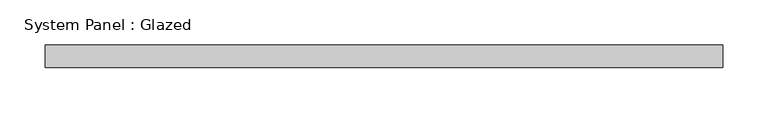
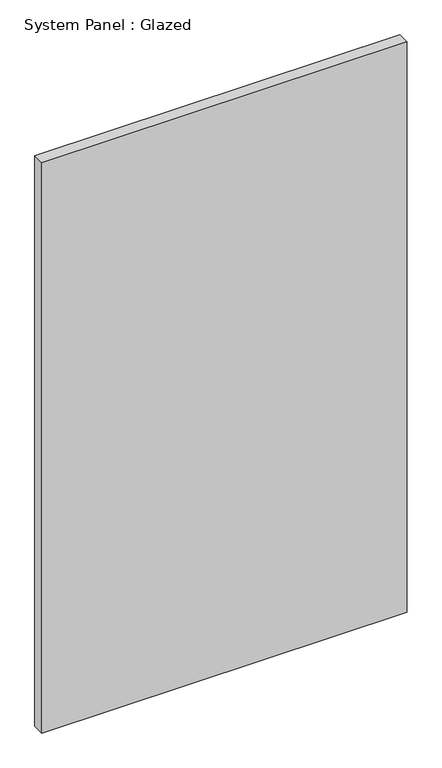
"""IFC4 building model written with IfcOpenShell, lengths in millimetres: plate geometry, System Panel : Glazed."""

from ifc_helpers import new_model, si_unit, origin, origin_with_axes, place, context, project, spatial, polyline, outline, extrude, source, transform, mapped, element, save


def system_panel_glazed_12388ada(model_context):
    return source(origin(), model_context, "Body", "SweptSolid", [
        extrude(outline(polyline([(375.0, 24.5), (-375.0, 24.5), (-375.0, 49.5), (375.0, 49.5), (375.0, 24.5)])), origin_with_axes(), (0.0, 0.0, 1.0), 1237.5),
    ])


if __name__ == "__main__":
    model = new_model("IFC4")
    model_context = context("Model", 3, world=origin())
    ifc_project = project(units=[si_unit("LENGTHUNIT", "METRE", prefix="MILLI")], contexts=[model_context])
    site = spatial("IfcSite", under=ifc_project)
    building = spatial("IfcBuilding", under=site)
    placement = place(None, origin())
    system_panel_glazed_shape = system_panel_glazed_12388ada(model_context)
    element("IfcPlate", 1, ObjectType="System Panel : Glazed", at=placement, inside=building, context=model_context, shape_type="MappedRepresentation", body=[
        mapped(system_panel_glazed_shape, transform((0.0, 0.0, 0.0), x_axis=(1.0, 0.0, 0.0), y_axis=(0.0, 1.0, 0.0), z_axis=(0.0, 0.0, 1.0))),
    ])
    save(model, "model.ifc")

# Revit data of these elements
# Element 1 (IfcPlate, "System Panel : Glazed")
#   Materials on its faces: "Glass"
# Materials
#   "Glass": class "Glass", colour RGB 218 227 224, transparency 0.85, Description = "Soda Lime Glass", Cost = 0
